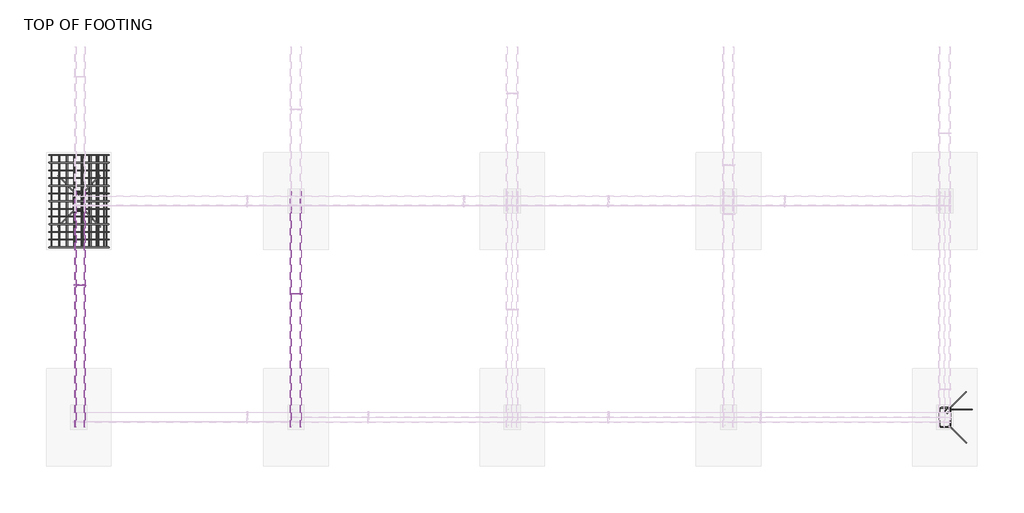
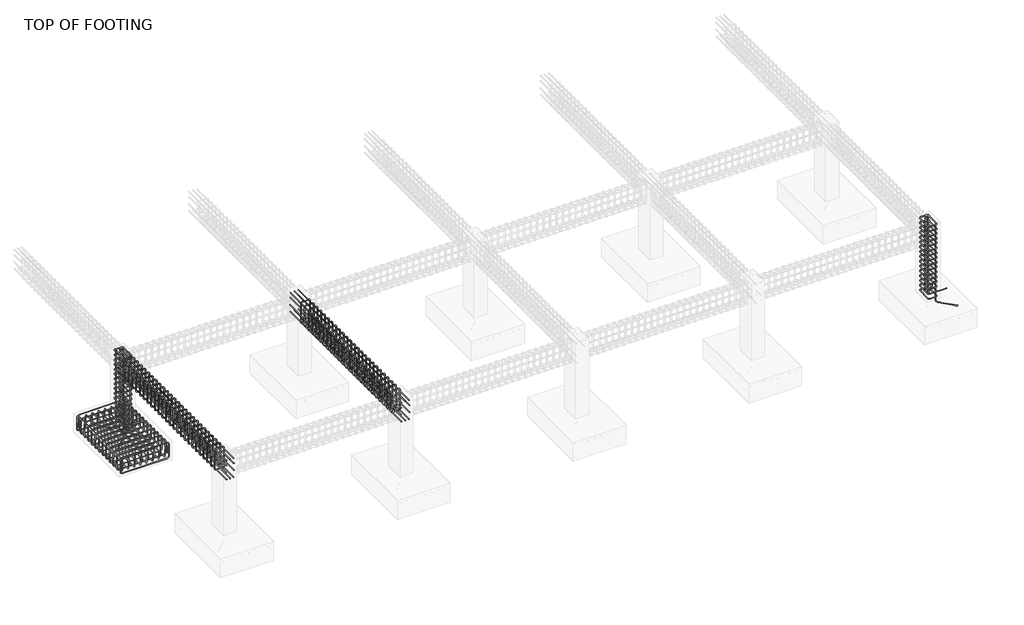
# One storey, part 5 of 21: 28 reinforcing bars.
"""IFC4 building model written with IfcOpenShell, lengths in millimetres."""

from ifc_helpers import new_model, si_unit, point, frame, origin, place, context, project, spatial, polyline, circle_curve, trimmed, segment, composite_curve, source, transform, mapped, element, save
from ifc_brep_helpers import swept_disk

model = new_model("IFC4")

# Units and contexts
model_context = context("Model", 3, world=origin())
ifc_project = project(units=[si_unit("LENGTHUNIT", "METRE", prefix="MILLI")], contexts=[model_context])

# Site, building, storey
site = spatial("IfcSite", under=ifc_project)
building = spatial("IfcBuilding", under=site)
storey = spatial("IfcBuildingStorey", under=building, Name="TOP OF FOOTING", Elevation=-1828.8)

# Reinforcing bars
placement = place(None, origin())
reinforcing_bar_shape = source(origin(), model_context, "Body", "SolidModel", [
    swept_disk(composite_curve([segment(polyline([(-13268.2584825, 4443.1886958, -2045.4168622), (-13268.2584825, 4443.1886958, -2192.7168622)]), True, "CONTINUOUS"), segment(trimmed(circle_curve(frame((-13314.6084825, 4443.1886958, -2192.7168622), z_axis=(0.0, 1.0, 0.0), x_axis=(46.350000000000364, 0.0, 0.0)), 46.35), [point((-13268.2584825, 4443.1886958, -2192.7168622))], [point((-13314.6084825, 4443.1886958, -2239.0668622))], True, "CARTESIAN"), True, "CONTINUOUS"), segment(polyline([(-13314.6084825, 4443.1886958, -2239.0668622), (-14329.2084825, 4443.1886958, -2239.0668622)]), True, "CONTINUOUS"), segment(trimmed(circle_curve(frame((-14329.2084825, 4443.1886958, -2192.7168622), z_axis=(0.0, 1.0, 0.0), x_axis=(0.0, 0.0, -46.34999999999991)), 46.35), [point((-14329.2084825, 4443.1886958, -2239.0668622))], [point((-14375.5584825, 4443.1886958, -2192.7168622))], True, "CARTESIAN"), True, "CONTINUOUS"), segment(polyline([(-14375.5584825, 4443.1886958, -2192.7168622), (-14375.5584825, 4443.1886958, -2045.4168622)]), True, "CONTINUOUS")], self_intersect=False), 6.35),
])
element("IfcReinforcingBar", 1, at=placement, inside=storey, context=model_context, shape_type="MappedRepresentation", body=[
    mapped(reinforcing_bar_shape, transform((0.0, 0.0, 0.0), x_axis=(1.0, 0.0, 0.0), y_axis=(0.0, 1.0, 0.0), z_axis=(0.0, 0.0, 1.0))),
    mapped(reinforcing_bar_shape, transform((0.0, -142.275, 0.0), x_axis=(1.0, 0.0, 0.0), y_axis=(0.0, 1.0, 0.0), z_axis=(0.0, 0.0, 1.0))),
    mapped(reinforcing_bar_shape, transform((0.0, -284.55, 0.0), x_axis=(1.0, 0.0, 0.0), y_axis=(0.0, 1.0, 0.0), z_axis=(0.0, 0.0, 1.0))),
    mapped(reinforcing_bar_shape, transform((0.0, -426.825, 0.0), x_axis=(1.0, 0.0, 0.0), y_axis=(0.0, 1.0, 0.0), z_axis=(0.0, 0.0, 1.0))),
    mapped(reinforcing_bar_shape, transform((0.0, -569.1, 0.0), x_axis=(1.0, 0.0, 0.0), y_axis=(0.0, 1.0, 0.0), z_axis=(0.0, 0.0, 1.0))),
    mapped(reinforcing_bar_shape, transform((0.0, -711.375, 0.0), x_axis=(1.0, 0.0, 0.0), y_axis=(0.0, 1.0, 0.0), z_axis=(0.0, 0.0, 1.0))),
    mapped(reinforcing_bar_shape, transform((0.0, -853.65, 0.0), x_axis=(1.0, 0.0, 0.0), y_axis=(0.0, 1.0, 0.0), z_axis=(0.0, 0.0, 1.0))),
    mapped(reinforcing_bar_shape, transform((0.0, -995.925, 0.0), x_axis=(1.0, 0.0, 0.0), y_axis=(0.0, 1.0, 0.0), z_axis=(0.0, 0.0, 1.0))),
    mapped(reinforcing_bar_shape, transform((0.0, -1138.2, 0.0), x_axis=(1.0, 0.0, 0.0), y_axis=(0.0, 1.0, 0.0), z_axis=(0.0, 0.0, 1.0))),
    mapped(reinforcing_bar_shape, transform((0.0, -1280.475, 0.0), x_axis=(1.0, 0.0, 0.0), y_axis=(0.0, 1.0, 0.0), z_axis=(0.0, 0.0, 1.0))),
    mapped(reinforcing_bar_shape, transform((0.0, -1422.75, 0.0), x_axis=(1.0, 0.0, 0.0), y_axis=(0.0, 1.0, 0.0), z_axis=(0.0, 0.0, 1.0))),
    mapped(reinforcing_bar_shape, transform((0.0, -1565.025, 0.0), x_axis=(1.0, 0.0, 0.0), y_axis=(0.0, 1.0, 0.0), z_axis=(0.0, 0.0, 1.0))),
    mapped(reinforcing_bar_shape, transform((0.0, -1707.3, 0.0), x_axis=(1.0, 0.0, 0.0), y_axis=(0.0, 1.0, 0.0), z_axis=(0.0, 0.0, 1.0))),
])
reinforcing_bar_2_shape = source(origin(), model_context, "Body", "SolidModel", [
    swept_disk(composite_curve([segment(polyline([(-14372.2274202, 4443.1886958, -2057.1074344), (-14372.2274202, 4443.1886958, -1909.8074344)]), True, "CONTINUOUS"), segment(trimmed(circle_curve(frame((-14325.8774202, 4443.1886958, -1909.8074344), z_axis=(0.0, 1.0, 0.0), x_axis=(-46.350000000000364, 0.0, 0.0)), 46.35), [point((-14372.2274202, 4443.1886958, -1909.8074344))], [point((-14325.8774202, 4443.1886958, -1863.4574344))], True, "CARTESIAN"), True, "CONTINUOUS"), segment(polyline([(-14325.8774202, 4443.1886958, -1863.4574344), (-13316.98705, 4443.1886958, -1863.4574344)]), True, "CONTINUOUS"), segment(trimmed(circle_curve(frame((-13316.98705, 4443.1886958, -1909.8074344), z_axis=(0.0, 1.0, 0.0), x_axis=(0.0, 0.0, 46.34999999999991)), 46.35), [point((-13316.98705, 4443.1886958, -1863.4574344))], [point((-13270.63705, 4443.1886958, -1909.8074344))], True, "CARTESIAN"), True, "CONTINUOUS"), segment(polyline([(-13270.63705, 4443.1886958, -1909.8074344), (-13270.63705, 4443.1886958, -2057.1074344)]), True, "CONTINUOUS")], self_intersect=False), 6.35),
])
element("IfcReinforcingBar", 2, at=placement, inside=storey, context=model_context, shape_type="MappedRepresentation", body=[
    mapped(reinforcing_bar_2_shape, transform((0.0, 0.0, 0.0), x_axis=(1.0, 0.0, 0.0), y_axis=(0.0, 1.0, 0.0), z_axis=(0.0, 0.0, 1.0))),
    mapped(reinforcing_bar_2_shape, transform((0.0, -142.275, 0.0), x_axis=(1.0, 0.0, 0.0), y_axis=(0.0, 1.0, 0.0), z_axis=(0.0, 0.0, 1.0))),
    mapped(reinforcing_bar_2_shape, transform((0.0, -284.55, 0.0), x_axis=(1.0, 0.0, 0.0), y_axis=(0.0, 1.0, 0.0), z_axis=(0.0, 0.0, 1.0))),
    mapped(reinforcing_bar_2_shape, transform((0.0, -426.825, 0.0), x_axis=(1.0, 0.0, 0.0), y_axis=(0.0, 1.0, 0.0), z_axis=(0.0, 0.0, 1.0))),
    mapped(reinforcing_bar_2_shape, transform((0.0, -569.1, 0.0), x_axis=(1.0, 0.0, 0.0), y_axis=(0.0, 1.0, 0.0), z_axis=(0.0, 0.0, 1.0))),
    mapped(reinforcing_bar_2_shape, transform((0.0, -711.375, 0.0), x_axis=(1.0, 0.0, 0.0), y_axis=(0.0, 1.0, 0.0), z_axis=(0.0, 0.0, 1.0))),
    mapped(reinforcing_bar_2_shape, transform((0.0, -853.65, 0.0), x_axis=(1.0, 0.0, 0.0), y_axis=(0.0, 1.0, 0.0), z_axis=(0.0, 0.0, 1.0))),
    mapped(reinforcing_bar_2_shape, transform((0.0, -995.925, 0.0), x_axis=(1.0, 0.0, 0.0), y_axis=(0.0, 1.0, 0.0), z_axis=(0.0, 0.0, 1.0))),
    mapped(reinforcing_bar_2_shape, transform((0.0, -1138.2, 0.0), x_axis=(1.0, 0.0, 0.0), y_axis=(0.0, 1.0, 0.0), z_axis=(0.0, 0.0, 1.0))),
    mapped(reinforcing_bar_2_shape, transform((0.0, -1280.475, 0.0), x_axis=(1.0, 0.0, 0.0), y_axis=(0.0, 1.0, 0.0), z_axis=(0.0, 0.0, 1.0))),
    mapped(reinforcing_bar_2_shape, transform((0.0, -1422.75, 0.0), x_axis=(1.0, 0.0, 0.0), y_axis=(0.0, 1.0, 0.0), z_axis=(0.0, 0.0, 1.0))),
    mapped(reinforcing_bar_2_shape, transform((0.0, -1565.025, 0.0), x_axis=(1.0, 0.0, 0.0), y_axis=(0.0, 1.0, 0.0), z_axis=(0.0, 0.0, 1.0))),
    mapped(reinforcing_bar_2_shape, transform((0.0, -1707.3, 0.0), x_axis=(1.0, 0.0, 0.0), y_axis=(0.0, 1.0, 0.0), z_axis=(0.0, 0.0, 1.0))),
])
reinforcing_bar_3_shape = source(origin(), model_context, "Body", "SolidModel", [
    swept_disk(composite_curve([segment(polyline([(-13314.2120502, 4443.1886958, -2099.3509187), (-13314.2120502, 4443.1886958, -1952.0509187)]), True, "CONTINUOUS"), segment(trimmed(circle_curve(frame((-13314.2120502, 4396.8386958, -1952.0509187), z_axis=(1.0, 0.0, 0.0), x_axis=(0.0, 46.349999999999454, 0.0)), 46.35), [point((-13314.2120502, 4443.1886958, -1952.0509187))], [point((-13314.2120502, 4396.8386958, -1905.7009187))], True, "CARTESIAN"), True, "CONTINUOUS"), segment(polyline([(-13314.2120502, 4396.8386958, -1905.7009187), (-13314.2120502, 2782.2386958, -1905.7009187)]), True, "CONTINUOUS"), segment(trimmed(circle_curve(frame((-13314.2120502, 2782.2386958, -1952.0509187), z_axis=(1.0, 0.0, 0.0), x_axis=(0.0, 0.0, 46.34999999999991)), 46.35), [point((-13314.2120502, 2782.2386958, -1905.7009187))], [point((-13314.2120502, 2735.8886958, -1952.0509187))], True, "CARTESIAN"), True, "CONTINUOUS"), segment(polyline([(-13314.2120502, 2735.8886958, -1952.0509187), (-13314.2120502, 2735.8886958, -2099.3509187)]), True, "CONTINUOUS")], self_intersect=False), 6.35),
])
element("IfcReinforcingBar", 3, at=placement, inside=storey, context=model_context, shape_type="MappedRepresentation", body=[
    mapped(reinforcing_bar_3_shape, transform((0.0, 0.0, 0.0), x_axis=(1.0, 0.0, 0.0), y_axis=(0.0, 1.0, 0.0), z_axis=(0.0, 0.0, 1.0))),
    mapped(reinforcing_bar_3_shape, transform((-145.0295561, 0.0, 0.0), x_axis=(1.0, 0.0, 0.0), y_axis=(0.0, 1.0, 0.0), z_axis=(0.0, 0.0, 1.0))),
    mapped(reinforcing_bar_3_shape, transform((-290.0591123, 0.0, 0.0), x_axis=(1.0, 0.0, 0.0), y_axis=(0.0, 1.0, 0.0), z_axis=(0.0, 0.0, 1.0))),
    mapped(reinforcing_bar_3_shape, transform((-435.0886684, 0.0, 0.0), x_axis=(1.0, 0.0, 0.0), y_axis=(0.0, 1.0, 0.0), z_axis=(0.0, 0.0, 1.0))),
    mapped(reinforcing_bar_3_shape, transform((-580.1182245, 0.0, 0.0), x_axis=(1.0, 0.0, 0.0), y_axis=(0.0, 1.0, 0.0), z_axis=(0.0, 0.0, 1.0))),
    mapped(reinforcing_bar_3_shape, transform((-725.1477807, 0.0, 0.0), x_axis=(1.0, 0.0, 0.0), y_axis=(0.0, 1.0, 0.0), z_axis=(0.0, 0.0, 1.0))),
    mapped(reinforcing_bar_3_shape, transform((-870.1773368, 0.0, 0.0), x_axis=(1.0, 0.0, 0.0), y_axis=(0.0, 1.0, 0.0), z_axis=(0.0, 0.0, 1.0))),
    mapped(reinforcing_bar_3_shape, transform((-1015.206893, 0.0, 0.0), x_axis=(1.0, 0.0, 0.0), y_axis=(0.0, 1.0, 0.0), z_axis=(0.0, 0.0, 1.0))),
])
reinforcing_bar_4_shape = source(origin(), model_context, "Body", "SolidModel", [
    swept_disk(composite_curve([segment(polyline([(-14329.4189432, 4443.1886958, -2006.0306816), (-14329.4189432, 4443.1886958, -2153.3306816)]), True, "CONTINUOUS"), segment(trimmed(circle_curve(frame((-14329.4189432, 4396.8386958, -2153.3306816), z_axis=(-1.0, 0.0, 0.0), x_axis=(0.0, 46.349999999999454, 0.0)), 46.35), [point((-14329.4189432, 4443.1886958, -2153.3306816))], [point((-14329.4189432, 4396.8386958, -2199.6806816))], True, "CARTESIAN"), True, "CONTINUOUS"), segment(polyline([(-14329.4189432, 4396.8386958, -2199.6806816), (-14329.4189432, 2782.2386958, -2199.6806816)]), True, "CONTINUOUS"), segment(trimmed(circle_curve(frame((-14329.4189432, 2782.2386958, -2153.3306816), z_axis=(-1.0, 0.0, 0.0), x_axis=(0.0, 0.0, -46.34999999999991)), 46.35), [point((-14329.4189432, 2782.2386958, -2199.6806816))], [point((-14329.4189432, 2735.8886958, -2153.3306816))], True, "CARTESIAN"), True, "CONTINUOUS"), segment(polyline([(-14329.4189432, 2735.8886958, -2153.3306816), (-14329.4189432, 2735.8886958, -2006.0306816)]), True, "CONTINUOUS")], self_intersect=False), 6.35),
])
element("IfcReinforcingBar", 4, at=placement, inside=storey, context=model_context, shape_type="MappedRepresentation", body=[
    mapped(reinforcing_bar_4_shape, transform((0.0, 0.0, 0.0), x_axis=(1.0, 0.0, 0.0), y_axis=(0.0, 1.0, 0.0), z_axis=(0.0, 0.0, 1.0))),
    mapped(reinforcing_bar_4_shape, transform((138.8823255, 0.0, 0.0), x_axis=(1.0, 0.0, 0.0), y_axis=(0.0, 1.0, 0.0), z_axis=(0.0, 0.0, 1.0))),
    mapped(reinforcing_bar_4_shape, transform((277.7646509, 0.0, 0.0), x_axis=(1.0, 0.0, 0.0), y_axis=(0.0, 1.0, 0.0), z_axis=(0.0, 0.0, 1.0))),
    mapped(reinforcing_bar_4_shape, transform((416.6469764, 0.0, 0.0), x_axis=(1.0, 0.0, 0.0), y_axis=(0.0, 1.0, 0.0), z_axis=(0.0, 0.0, 1.0))),
    mapped(reinforcing_bar_4_shape, transform((555.5293018, 0.0, 0.0), x_axis=(1.0, 0.0, 0.0), y_axis=(0.0, 1.0, 0.0), z_axis=(0.0, 0.0, 1.0))),
    mapped(reinforcing_bar_4_shape, transform((694.4116273, 0.0, 0.0), x_axis=(1.0, 0.0, 0.0), y_axis=(0.0, 1.0, 0.0), z_axis=(0.0, 0.0, 1.0))),
    mapped(reinforcing_bar_4_shape, transform((833.2939527, 0.0, 0.0), x_axis=(1.0, 0.0, 0.0), y_axis=(0.0, 1.0, 0.0), z_axis=(0.0, 0.0, 1.0))),
    mapped(reinforcing_bar_4_shape, transform((972.1762782, 0.0, 0.0), x_axis=(1.0, 0.0, 0.0), y_axis=(0.0, 1.0, 0.0), z_axis=(0.0, 0.0, 1.0))),
])
reinforcing_bar_5_shape = source(origin(), model_context, "Body", "SolidModel", [
    swept_disk(composite_curve([segment(polyline([(-13827.5198431, 3703.2629305, -46.35), (-13771.7762801, 3759.0064934, -46.35)]), True, "CONTINUOUS"), segment(trimmed(circle_curve(frame((-13749.6084825, 3736.8386958, -46.35), z_axis=(0.0, 0.0, -1.0), x_axis=(-22.167797600000995, 22.167797600000085, 0.0)), 31.35), [point((-13771.7762801, 3759.0064934, -46.35))], [point((-13718.2584825, 3736.8386958, -46.35))], True, "CARTESIAN"), True, "CONTINUOUS"), segment(polyline([(-13718.2584825, 3736.8386958, -46.35), (-13718.2584825, 3442.2386958, -46.35)]), True, "CONTINUOUS"), segment(trimmed(circle_curve(frame((-13749.6084825, 3442.2386958, -46.35), z_axis=(0.0, 0.0, -1.0), x_axis=(31.350000000000364, 0.0, 0.0)), 31.35), [point((-13718.2584825, 3442.2386958, -46.35))], [point((-13749.6084825, 3410.8886958, -46.35))], True, "CARTESIAN"), True, "CONTINUOUS"), segment(polyline([(-13749.6084825, 3410.8886958, -46.35), (-13894.2084825, 3410.8886958, -46.35)]), True, "CONTINUOUS"), segment(trimmed(circle_curve(frame((-13894.2084825, 3442.2189107, -45.2363875), z_axis=(0.0, 0.035521928334481916, -0.9993688971583016), x_axis=(0.0, -31.3302149000001, -1.1136125000000021)), 31.35), [point((-13894.2084825, 3410.8886958, -46.35))], [point((-13925.5584825, 3442.2189107, -45.2363875))], True, "CARTESIAN"), True, "CONTINUOUS"), segment(polyline([(-13925.5584825, 3442.2189107, -45.2363875), (-13925.5584825, 3736.8584809, -34.7636125)]), True, "CONTINUOUS"), segment(trimmed(circle_curve(frame((-13894.2084825, 3736.8584809, -34.7636125), z_axis=(0.0, 0.035521928334481916, -0.9993688971583016), x_axis=(-31.350000000000364, 0.0, 0.0)), 31.35), [point((-13925.5584825, 3736.8584809, -34.7636125))], [point((-13894.2084825, 3768.1886958, -33.65))], True, "CARTESIAN"), True, "CONTINUOUS"), segment(polyline([(-13894.2084825, 3768.1886958, -33.65), (-13749.6084825, 3768.1886958, -33.65)]), True, "CONTINUOUS"), segment(trimmed(circle_curve(frame((-13749.6084825, 3736.8386958, -33.65), z_axis=(0.0, 0.0, -1.0), x_axis=(0.0, 31.34999999999991, 0.0)), 31.35), [point((-13749.6084825, 3768.1886958, -33.65))], [point((-13727.4406849, 3714.6708982, -33.65))], True, "CARTESIAN"), True, "CONTINUOUS"), segment(polyline([(-13727.4406849, 3714.6708982, -33.65), (-13783.1842479, 3658.9273353, -33.65)]), True, "CONTINUOUS")], self_intersect=False), 6.35),
])
element("IfcReinforcingBar", 5, at=placement, inside=storey, context=model_context, shape_type="MappedRepresentation", body=[
    mapped(reinforcing_bar_5_shape, transform((0.0, 0.0, 0.0), x_axis=(1.0, 0.0, 0.0), y_axis=(0.0, 1.0, 0.0), z_axis=(0.0, 0.0, 1.0))),
    mapped(reinforcing_bar_5_shape, transform((0.0, 0.0, -115.74), x_axis=(1.0, 0.0, 0.0), y_axis=(0.0, 1.0, 0.0), z_axis=(0.0, 0.0, 1.0))),
    mapped(reinforcing_bar_5_shape, transform((0.0, 0.0, -231.48), x_axis=(1.0, 0.0, 0.0), y_axis=(0.0, 1.0, 0.0), z_axis=(0.0, 0.0, 1.0))),
    mapped(reinforcing_bar_5_shape, transform((0.0, 0.0, -347.22), x_axis=(1.0, 0.0, 0.0), y_axis=(0.0, 1.0, 0.0), z_axis=(0.0, 0.0, 1.0))),
    mapped(reinforcing_bar_5_shape, transform((0.0, 0.0, -462.96), x_axis=(1.0, 0.0, 0.0), y_axis=(0.0, 1.0, 0.0), z_axis=(0.0, 0.0, 1.0))),
    mapped(reinforcing_bar_5_shape, transform((0.0, 0.0, -578.7), x_axis=(1.0, 0.0, 0.0), y_axis=(0.0, 1.0, 0.0), z_axis=(0.0, 0.0, 1.0))),
    mapped(reinforcing_bar_5_shape, transform((0.0, 0.0, -694.44), x_axis=(1.0, 0.0, 0.0), y_axis=(0.0, 1.0, 0.0), z_axis=(0.0, 0.0, 1.0))),
    mapped(reinforcing_bar_5_shape, transform((0.0, 0.0, -810.18), x_axis=(1.0, 0.0, 0.0), y_axis=(0.0, 1.0, 0.0), z_axis=(0.0, 0.0, 1.0))),
    mapped(reinforcing_bar_5_shape, transform((0.0, 0.0, -925.92), x_axis=(1.0, 0.0, 0.0), y_axis=(0.0, 1.0, 0.0), z_axis=(0.0, 0.0, 1.0))),
    mapped(reinforcing_bar_5_shape, transform((0.0, 0.0, -1041.66), x_axis=(1.0, 0.0, 0.0), y_axis=(0.0, 1.0, 0.0), z_axis=(0.0, 0.0, 1.0))),
    mapped(reinforcing_bar_5_shape, transform((0.0, 0.0, -1157.4), x_axis=(1.0, 0.0, 0.0), y_axis=(0.0, 1.0, 0.0), z_axis=(0.0, 0.0, 1.0))),
    mapped(reinforcing_bar_5_shape, transform((0.0, 0.0, -1273.14), x_axis=(1.0, 0.0, 0.0), y_axis=(0.0, 1.0, 0.0), z_axis=(0.0, 0.0, 1.0))),
    mapped(reinforcing_bar_5_shape, transform((0.0, 0.0, -1388.88), x_axis=(1.0, 0.0, 0.0), y_axis=(0.0, 1.0, 0.0), z_axis=(0.0, 0.0, 1.0))),
    mapped(reinforcing_bar_5_shape, transform((0.0, 0.0, -1504.62), x_axis=(1.0, 0.0, 0.0), y_axis=(0.0, 1.0, 0.0), z_axis=(0.0, 0.0, 1.0))),
    mapped(reinforcing_bar_5_shape, transform((0.0, 0.0, -1620.36), x_axis=(1.0, 0.0, 0.0), y_axis=(0.0, 1.0, 0.0), z_axis=(0.0, 0.0, 1.0))),
    mapped(reinforcing_bar_5_shape, transform((0.0, 0.0, -1736.1), x_axis=(1.0, 0.0, 0.0), y_axis=(0.0, 1.0, 0.0), z_axis=(0.0, 0.0, 1.0))),
])
element("IfcReinforcingBar", 6, at=placement, inside=storey, context=model_context, shape_type="SolidModel", body=[
    swept_disk(composite_curve([segment(polyline([(-13750.0878823, 3737.940488, -40.0), (-13750.0878823, 3737.940488, -1882.5259187)]), True, "CONTINUOUS"), segment(trimmed(circle_curve(frame((-13703.7378823, 3737.940488, -1882.5259187), z_axis=(0.0, -1.0, 0.0), x_axis=(-46.350000000000364, 0.0, 0.0)), 46.35), [point((-13750.0878823, 3737.940488, -1882.5259187))], [point((-13703.7378823, 3737.940488, -1928.8759187))], True, "CARTESIAN"), True, "CONTINUOUS"), segment(polyline([(-13703.7378823, 3737.940488, -1928.8759187), (-13314.2120502, 3737.940488, -1928.8759187)]), True, "CONTINUOUS")], self_intersect=False), 6.35),
])
element("IfcReinforcingBar", 7, at=placement, inside=storey, context=model_context, shape_type="SolidModel", body=[
    swept_disk(composite_curve([segment(polyline([(-13750.0878823, 3737.940488, -40.0), (-13750.0878823, 3737.940488, -1882.5259187)]), True, "CONTINUOUS"), segment(trimmed(circle_curve(frame((-13717.6297647, 3771.0281458, -1882.5259187), z_axis=(0.7138653253877265, -0.7002830122236834, 0.0), x_axis=(-32.45811760000106, -33.08765779999976, 0.0)), 46.35), [point((-13750.0878823, 3737.940488, -1882.5259187))], [point((-13717.6297647, 3771.0281458, -1928.8759187))], True, "CARTESIAN"), True, "CONTINUOUS"), segment(polyline([(-13717.6297647, 3771.0281458, -1928.8759187), (-13432.8602442, 4061.320903, -1928.8759187)]), True, "CONTINUOUS")], self_intersect=False), 6.35),
])
element("IfcReinforcingBar", 8, at=placement, inside=storey, context=model_context, shape_type="SolidModel", body=[
    swept_disk(composite_curve([segment(polyline([(-13893.7290828, 3737.940488, -40.0), (-13893.7290828, 3737.940488, -1882.5259187)]), True, "CONTINUOUS"), segment(trimmed(circle_curve(frame((-13926.1872004, 3771.0281458, -1882.5259187), z_axis=(0.7138653253877091, 0.700283012223701, 0.0), x_axis=(32.45811759999924, -33.08765779999976, 0.0)), 46.35), [point((-13893.7290828, 3737.940488, -1882.5259187))], [point((-13926.1872004, 3771.0281458, -1928.8759187))], True, "CARTESIAN"), True, "CONTINUOUS"), segment(polyline([(-13926.1872004, 3771.0281458, -1928.8759187), (-14210.9567208, 4061.320903, -1928.8759187)]), True, "CONTINUOUS")], self_intersect=False), 6.35),
])
element("IfcReinforcingBar", 9, at=placement, inside=storey, context=model_context, shape_type="SolidModel", body=[
    swept_disk(composite_curve([segment(polyline([(-13745.0878823, 3438.6369036, -40.0), (-13745.0878823, 3438.6369036, -1882.5259187)]), True, "CONTINUOUS"), segment(trimmed(circle_curve(frame((-13712.6297647, 3405.5492458, -1882.5259187), z_axis=(-0.7138653253877265, -0.7002830122236834, 0.0), x_axis=(-32.45811760000106, 33.087657800000216, 0.0)), 46.35), [point((-13745.0878823, 3438.6369036, -1882.5259187))], [point((-13712.6297647, 3405.5492458, -1928.8759187))], True, "CARTESIAN"), True, "CONTINUOUS"), segment(polyline([(-13712.6297647, 3405.5492458, -1928.8759187), (-13427.8602442, 3115.2564887, -1928.8759187)]), True, "CONTINUOUS")], self_intersect=False), 6.35),
])
element("IfcReinforcingBar", 10, at=placement, inside=storey, context=model_context, shape_type="SolidModel", body=[
    swept_disk(composite_curve([segment(polyline([(-13893.7290828, 3441.1369036, -40.0), (-13893.7290828, 3441.1369036, -1882.5259187)]), True, "CONTINUOUS"), segment(trimmed(circle_curve(frame((-13926.1872004, 3408.0492458, -1882.5259187), z_axis=(-0.7138653253877092, 0.7002830122237009, 0.0), x_axis=(32.45811759999924, 33.087657800000216, 0.0)), 46.35), [point((-13893.7290828, 3441.1369036, -1882.5259187))], [point((-13926.1872004, 3408.0492458, -1928.8759187))], True, "CARTESIAN"), True, "CONTINUOUS"), segment(polyline([(-13926.1872004, 3408.0492458, -1928.8759187), (-14210.9567208, 3117.7564887, -1928.8759187)]), True, "CONTINUOUS")], self_intersect=False), 6.35),
])
reinforcing_bar_6_shape = source(origin(), model_context, "Body", "SolidModel", [
    swept_disk(composite_curve([segment(polyline([(2192.2072855, -296.7370695, -46.35), (2247.9508485, -240.9935066, -46.35)]), True, "CONTINUOUS"), segment(trimmed(circle_curve(frame((2270.1186461, -263.1613042, -46.35), z_axis=(0.0, 0.0, -1.0), x_axis=(-22.167797600000085, 22.16779760000003, 0.0)), 31.35), [point((2247.9508485, -240.9935066, -46.35))], [point((2301.4686461, -263.1613042, -46.35))], True, "CARTESIAN"), True, "CONTINUOUS"), segment(polyline([(2301.4686461, -263.1613042, -46.35), (2301.4686461, -557.7613042, -46.35)]), True, "CONTINUOUS"), segment(trimmed(circle_curve(frame((2270.1186461, -557.7613042, -46.35), z_axis=(0.0, 0.0, -1.0), x_axis=(31.34999999999991, 0.0, 0.0)), 31.35), [point((2301.4686461, -557.7613042, -46.35))], [point((2270.1186461, -589.1113042, -46.35))], True, "CARTESIAN"), True, "CONTINUOUS"), segment(polyline([(2270.1186461, -589.1113042, -46.35), (2125.5186461, -589.1113042, -46.35)]), True, "CONTINUOUS"), segment(trimmed(circle_curve(frame((2125.5186461, -557.7810893, -45.2363875), z_axis=(0.0, 0.035521928334481916, -0.9993688971583016), x_axis=(0.0, -31.330214899999987, -1.1136125000000021)), 31.35), [point((2125.5186461, -589.1113042, -46.35))], [point((2094.1686461, -557.7810893, -45.2363875))], True, "CARTESIAN"), True, "CONTINUOUS"), segment(polyline([(2094.1686461, -557.7810893, -45.2363875), (2094.1686461, -263.1415191, -34.7636125)]), True, "CONTINUOUS"), segment(trimmed(circle_curve(frame((2125.5186461, -263.1415191, -34.7636125), z_axis=(0.0, 0.035521928334481916, -0.9993688971583016), x_axis=(-31.34999999999991, 0.0, 0.0)), 31.35), [point((2094.1686461, -263.1415191, -34.7636125))], [point((2125.5186461, -231.8113042, -33.65))], True, "CARTESIAN"), True, "CONTINUOUS"), segment(polyline([(2125.5186461, -231.8113042, -33.65), (2270.1186461, -231.8113042, -33.65)]), True, "CONTINUOUS"), segment(trimmed(circle_curve(frame((2270.1186461, -263.1613042, -33.65), z_axis=(0.0, 0.0, -1.0), x_axis=(0.0, 31.350000000000023, 0.0)), 31.35), [point((2270.1186461, -231.8113042, -33.65))], [point((2292.2864437, -285.3291018, -33.65))], True, "CARTESIAN"), True, "CONTINUOUS"), segment(polyline([(2292.2864437, -285.3291018, -33.65), (2236.5428807, -341.0726647, -33.65)]), True, "CONTINUOUS")], self_intersect=False), 6.35),
])
element("IfcReinforcingBar", 11, at=placement, inside=storey, context=model_context, shape_type="MappedRepresentation", body=[
    mapped(reinforcing_bar_6_shape, transform((0.0, 0.0, 0.0), x_axis=(1.0, 0.0, 0.0), y_axis=(0.0, 1.0, 0.0), z_axis=(0.0, 0.0, 1.0))),
    mapped(reinforcing_bar_6_shape, transform((0.0, 0.0, -115.74), x_axis=(1.0, 0.0, 0.0), y_axis=(0.0, 1.0, 0.0), z_axis=(0.0, 0.0, 1.0))),
    mapped(reinforcing_bar_6_shape, transform((0.0, 0.0, -231.48), x_axis=(1.0, 0.0, 0.0), y_axis=(0.0, 1.0, 0.0), z_axis=(0.0, 0.0, 1.0))),
    mapped(reinforcing_bar_6_shape, transform((0.0, 0.0, -347.22), x_axis=(1.0, 0.0, 0.0), y_axis=(0.0, 1.0, 0.0), z_axis=(0.0, 0.0, 1.0))),
    mapped(reinforcing_bar_6_shape, transform((0.0, 0.0, -462.96), x_axis=(1.0, 0.0, 0.0), y_axis=(0.0, 1.0, 0.0), z_axis=(0.0, 0.0, 1.0))),
    mapped(reinforcing_bar_6_shape, transform((0.0, 0.0, -578.7), x_axis=(1.0, 0.0, 0.0), y_axis=(0.0, 1.0, 0.0), z_axis=(0.0, 0.0, 1.0))),
    mapped(reinforcing_bar_6_shape, transform((0.0, 0.0, -694.44), x_axis=(1.0, 0.0, 0.0), y_axis=(0.0, 1.0, 0.0), z_axis=(0.0, 0.0, 1.0))),
    mapped(reinforcing_bar_6_shape, transform((0.0, 0.0, -810.18), x_axis=(1.0, 0.0, 0.0), y_axis=(0.0, 1.0, 0.0), z_axis=(0.0, 0.0, 1.0))),
    mapped(reinforcing_bar_6_shape, transform((0.0, 0.0, -925.92), x_axis=(1.0, 0.0, 0.0), y_axis=(0.0, 1.0, 0.0), z_axis=(0.0, 0.0, 1.0))),
    mapped(reinforcing_bar_6_shape, transform((0.0, 0.0, -1041.66), x_axis=(1.0, 0.0, 0.0), y_axis=(0.0, 1.0, 0.0), z_axis=(0.0, 0.0, 1.0))),
    mapped(reinforcing_bar_6_shape, transform((0.0, 0.0, -1157.4), x_axis=(1.0, 0.0, 0.0), y_axis=(0.0, 1.0, 0.0), z_axis=(0.0, 0.0, 1.0))),
    mapped(reinforcing_bar_6_shape, transform((0.0, 0.0, -1273.14), x_axis=(1.0, 0.0, 0.0), y_axis=(0.0, 1.0, 0.0), z_axis=(0.0, 0.0, 1.0))),
    mapped(reinforcing_bar_6_shape, transform((0.0, 0.0, -1388.88), x_axis=(1.0, 0.0, 0.0), y_axis=(0.0, 1.0, 0.0), z_axis=(0.0, 0.0, 1.0))),
    mapped(reinforcing_bar_6_shape, transform((0.0, 0.0, -1504.62), x_axis=(1.0, 0.0, 0.0), y_axis=(0.0, 1.0, 0.0), z_axis=(0.0, 0.0, 1.0))),
    mapped(reinforcing_bar_6_shape, transform((0.0, 0.0, -1620.36), x_axis=(1.0, 0.0, 0.0), y_axis=(0.0, 1.0, 0.0), z_axis=(0.0, 0.0, 1.0))),
    mapped(reinforcing_bar_6_shape, transform((0.0, 0.0, -1736.1), x_axis=(1.0, 0.0, 0.0), y_axis=(0.0, 1.0, 0.0), z_axis=(0.0, 0.0, 1.0))),
])
element("IfcReinforcingBar", 12, at=placement, inside=storey, context=model_context, shape_type="SolidModel", body=[
    swept_disk(composite_curve([segment(polyline([(2269.6392463, -262.059512, -40.0), (2269.6392463, -262.059512, -1882.5259187)]), True, "CONTINUOUS"), segment(trimmed(circle_curve(frame((2315.9892463, -262.059512, -1882.5259187), z_axis=(0.0, -1.0, 0.0), x_axis=(-46.34999999999991, 0.0, 0.0)), 46.35), [point((2269.6392463, -262.059512, -1882.5259187))], [point((2315.9892463, -262.059512, -1928.8759187))], True, "CARTESIAN"), True, "CONTINUOUS"), segment(polyline([(2315.9892463, -262.059512, -1928.8759187), (2705.5150784, -262.059512, -1928.8759187)]), True, "CONTINUOUS")], self_intersect=False), 6.35),
])
element("IfcReinforcingBar", 13, at=placement, inside=storey, context=model_context, shape_type="SolidModel", body=[
    swept_disk(composite_curve([segment(polyline([(2269.6392463, -262.059512, -40.0), (2269.6392463, -262.059512, -1882.5259187)]), True, "CONTINUOUS"), segment(trimmed(circle_curve(frame((2302.0973639, -228.9718542, -1882.5259187), z_axis=(0.7138653253877265, -0.7002830122236834, 0.0), x_axis=(-32.458117599999696, -33.08765779999999, 0.0)), 46.35), [point((2269.6392463, -262.059512, -1882.5259187))], [point((2302.0973639, -228.9718542, -1928.8759187))], True, "CARTESIAN"), True, "CONTINUOUS"), segment(polyline([(2302.0973639, -228.9718542, -1928.8759187), (2586.8668844, 61.320903, -1928.8759187)]), True, "CONTINUOUS")], self_intersect=False), 6.35),
])
element("IfcReinforcingBar", 14, at=placement, inside=storey, context=model_context, shape_type="SolidModel", body=[
    swept_disk(composite_curve([segment(polyline([(2274.6392463, -561.3630964, -40.0), (2274.6392463, -561.3630964, -1882.5259187)]), True, "CONTINUOUS"), segment(trimmed(circle_curve(frame((2307.0973639, -594.4507542, -1882.5259187), z_axis=(-0.7138653253877265, -0.7002830122236834, 0.0), x_axis=(-32.458117599999696, 33.08765779999999, 0.0)), 46.35), [point((2274.6392463, -561.3630964, -1882.5259187))], [point((2307.0973639, -594.4507542, -1928.8759187))], True, "CARTESIAN"), True, "CONTINUOUS"), segment(polyline([(2307.0973639, -594.4507542, -1928.8759187), (2591.8668844, -884.7435113, -1928.8759187)]), True, "CONTINUOUS")], self_intersect=False), 6.35),
])
reinforcing_bar_7_shape = source(origin(), model_context, "Body", "SolidModel", [
    swept_disk(composite_curve([segment(polyline([(-13807.7927145, 3358.1886958, -488.7242346), (-13752.0491515, 3358.1886958, -544.4677976)]), True, "CONTINUOUS"), segment(trimmed(circle_curve(frame((-13729.8813539, 3358.1886958, -522.3), z_axis=(0.0, -1.0, 0.0), x_axis=(-22.167797599999176, 0.0, -22.167797600000085)), 31.35), [point((-13752.0491515, 3358.1886958, -544.4677976))], [point((-13698.5313539, 3358.1886958, -522.3))], True, "CARTESIAN"), True, "CONTINUOUS"), segment(polyline([(-13698.5313539, 3358.1886958, -522.3), (-13698.5313539, 3358.1886958, -77.7)]), True, "CONTINUOUS"), segment(trimmed(circle_curve(frame((-13729.8813539, 3358.1886958, -77.7), z_axis=(0.0, -1.0, 0.0), x_axis=(31.350000000000364, 0.0, 0.0)), 31.35), [point((-13698.5313539, 3358.1886958, -77.7))], [point((-13729.8813539, 3358.1886958, -46.35))], True, "CARTESIAN"), True, "CONTINUOUS"), segment(polyline([(-13729.8813539, 3358.1886958, -46.35), (-13874.4813539, 3358.1886958, -46.35)]), True, "CONTINUOUS"), segment(trimmed(circle_curve(frame((-13874.4813539, 3358.9732815, -77.6901807), z_axis=(0.0, -0.9996867842138424, -0.025026655153786322), x_axis=(0.0, -0.784585700000207, 31.340180699999998)), 31.35), [point((-13874.4813539, 3358.1886958, -46.35))], [point((-13905.8313539, 3358.9732815, -77.6901807))], True, "CARTESIAN"), True, "CONTINUOUS"), segment(polyline([(-13905.8313539, 3358.9732815, -77.6901807), (-13905.8313539, 3370.1041102, -522.3098193)]), True, "CONTINUOUS"), segment(trimmed(circle_curve(frame((-13874.4813539, 3370.1041102, -522.3098193), z_axis=(0.0, -0.9996867842138424, -0.025026655153786322), x_axis=(-31.349999999998545, 0.0, 0.0)), 31.35), [point((-13905.8313539, 3370.1041102, -522.3098193))], [point((-13874.4813539, 3370.8886958, -553.65))], True, "CARTESIAN"), True, "CONTINUOUS"), segment(polyline([(-13874.4813539, 3370.8886958, -553.65), (-13729.8813539, 3370.8886958, -553.65)]), True, "CONTINUOUS"), segment(trimmed(circle_curve(frame((-13729.8813539, 3370.8886958, -522.3), z_axis=(0.0, -1.0, 0.0), x_axis=(0.0, 0.0, -31.350000000000023)), 31.35), [point((-13729.8813539, 3370.8886958, -553.65))], [point((-13707.7135563, 3370.8886958, -500.1322024))], True, "CARTESIAN"), True, "CONTINUOUS"), segment(polyline([(-13707.7135563, 3370.8886958, -500.1322024), (-13763.4571193, 3370.8886958, -444.3886395)]), True, "CONTINUOUS")], self_intersect=False), 6.35),
])
element("IfcReinforcingBar", 15, at=placement, inside=storey, context=model_context, shape_type="MappedRepresentation", body=[
    mapped(reinforcing_bar_7_shape, transform((0.0, 0.0, 0.0), x_axis=(1.0, 0.0, 0.0), y_axis=(0.0, 1.0, 0.0), z_axis=(0.0, 0.0, 1.0))),
    mapped(reinforcing_bar_7_shape, transform((0.0, -147.3875, 0.0), x_axis=(1.0, 0.0, 0.0), y_axis=(0.0, 1.0, 0.0), z_axis=(0.0, 0.0, 1.0))),
    mapped(reinforcing_bar_7_shape, transform((0.0, -294.775, 0.0), x_axis=(1.0, 0.0, 0.0), y_axis=(0.0, 1.0, 0.0), z_axis=(0.0, 0.0, 1.0))),
    mapped(reinforcing_bar_7_shape, transform((0.0, -442.1625, 0.0), x_axis=(1.0, 0.0, 0.0), y_axis=(0.0, 1.0, 0.0), z_axis=(0.0, 0.0, 1.0))),
    mapped(reinforcing_bar_7_shape, transform((0.0, -589.55, 0.0), x_axis=(1.0, 0.0, 0.0), y_axis=(0.0, 1.0, 0.0), z_axis=(0.0, 0.0, 1.0))),
    mapped(reinforcing_bar_7_shape, transform((0.0, -736.9375, 0.0), x_axis=(1.0, 0.0, 0.0), y_axis=(0.0, 1.0, 0.0), z_axis=(0.0, 0.0, 1.0))),
    mapped(reinforcing_bar_7_shape, transform((0.0, -884.325, 0.0), x_axis=(1.0, 0.0, 0.0), y_axis=(0.0, 1.0, 0.0), z_axis=(0.0, 0.0, 1.0))),
    mapped(reinforcing_bar_7_shape, transform((0.0, -1031.7125, 0.0), x_axis=(1.0, 0.0, 0.0), y_axis=(0.0, 1.0, 0.0), z_axis=(0.0, 0.0, 1.0))),
    mapped(reinforcing_bar_7_shape, transform((0.0, -1179.1, 0.0), x_axis=(1.0, 0.0, 0.0), y_axis=(0.0, 1.0, 0.0), z_axis=(0.0, 0.0, 1.0))),
    mapped(reinforcing_bar_7_shape, transform((0.0, -1326.4875, 0.0), x_axis=(1.0, 0.0, 0.0), y_axis=(0.0, 1.0, 0.0), z_axis=(0.0, 0.0, 1.0))),
    mapped(reinforcing_bar_7_shape, transform((0.0, -1473.875, 0.0), x_axis=(1.0, 0.0, 0.0), y_axis=(0.0, 1.0, 0.0), z_axis=(0.0, 0.0, 1.0))),
    mapped(reinforcing_bar_7_shape, transform((0.0, -1621.2625, 0.0), x_axis=(1.0, 0.0, 0.0), y_axis=(0.0, 1.0, 0.0), z_axis=(0.0, 0.0, 1.0))),
    mapped(reinforcing_bar_7_shape, transform((0.0, -1768.65, 0.0), x_axis=(1.0, 0.0, 0.0), y_axis=(0.0, 1.0, 0.0), z_axis=(0.0, 0.0, 1.0))),
    mapped(reinforcing_bar_7_shape, transform((0.0, -1916.0375, 0.0), x_axis=(1.0, 0.0, 0.0), y_axis=(0.0, 1.0, 0.0), z_axis=(0.0, 0.0, 1.0))),
    mapped(reinforcing_bar_7_shape, transform((0.0, -2063.425, 0.0), x_axis=(1.0, 0.0, 0.0), y_axis=(0.0, 1.0, 0.0), z_axis=(0.0, 0.0, 1.0))),
    mapped(reinforcing_bar_7_shape, transform((0.0, -2210.8125, 0.0), x_axis=(1.0, 0.0, 0.0), y_axis=(0.0, 1.0, 0.0), z_axis=(0.0, 0.0, 1.0))),
    mapped(reinforcing_bar_7_shape, transform((0.0, -2358.2, 0.0), x_axis=(1.0, 0.0, 0.0), y_axis=(0.0, 1.0, 0.0), z_axis=(0.0, 0.0, 1.0))),
    mapped(reinforcing_bar_7_shape, transform((0.0, -2505.5875, 0.0), x_axis=(1.0, 0.0, 0.0), y_axis=(0.0, 1.0, 0.0), z_axis=(0.0, 0.0, 1.0))),
    mapped(reinforcing_bar_7_shape, transform((0.0, -2652.975, 0.0), x_axis=(1.0, 0.0, 0.0), y_axis=(0.0, 1.0, 0.0), z_axis=(0.0, 0.0, 1.0))),
    mapped(reinforcing_bar_7_shape, transform((0.0, -2800.3625, 0.0), x_axis=(1.0, 0.0, 0.0), y_axis=(0.0, 1.0, 0.0), z_axis=(0.0, 0.0, 1.0))),
    mapped(reinforcing_bar_7_shape, transform((0.0, -2947.75, 0.0), x_axis=(1.0, 0.0, 0.0), y_axis=(0.0, 1.0, 0.0), z_axis=(0.0, 0.0, 1.0))),
    mapped(reinforcing_bar_7_shape, transform((0.0, -3095.1375, 0.0), x_axis=(1.0, 0.0, 0.0), y_axis=(0.0, 1.0, 0.0), z_axis=(0.0, 0.0, 1.0))),
    mapped(reinforcing_bar_7_shape, transform((0.0, -3242.525, 0.0), x_axis=(1.0, 0.0, 0.0), y_axis=(0.0, 1.0, 0.0), z_axis=(0.0, 0.0, 1.0))),
    mapped(reinforcing_bar_7_shape, transform((0.0, -3389.9125, 0.0), x_axis=(1.0, 0.0, 0.0), y_axis=(0.0, 1.0, 0.0), z_axis=(0.0, 0.0, 1.0))),
    mapped(reinforcing_bar_7_shape, transform((0.0, -3537.3, 0.0), x_axis=(1.0, 0.0, 0.0), y_axis=(0.0, 1.0, 0.0), z_axis=(0.0, 0.0, 1.0))),
])
reinforcing_bar_8_shape = source(origin(), model_context, "Body", "SolidModel", [
    swept_disk(composite_curve([segment(polyline([(-13722.3514306, 3774.5386958, -70.2), (-13722.3514306, -595.4613042, -70.2)]), True, "CONTINUOUS")], self_intersect=False), 6.35),
])
element("IfcReinforcingBar", 16, at=placement, inside=storey, context=model_context, shape_type="MappedRepresentation", body=[
    mapped(reinforcing_bar_8_shape, transform((0.0, 0.0, 0.0), x_axis=(1.0, 0.0, 0.0), y_axis=(0.0, 1.0, 0.0), z_axis=(0.0, 0.0, 1.0))),
    mapped(reinforcing_bar_8_shape, transform((-77.925124, 0.0, 0.0), x_axis=(1.0, 0.0, 0.0), y_axis=(0.0, 1.0, 0.0), z_axis=(0.0, 0.0, 1.0))),
    mapped(reinforcing_bar_8_shape, transform((-155.850248, 0.0, 0.0), x_axis=(1.0, 0.0, 0.0), y_axis=(0.0, 1.0, 0.0), z_axis=(0.0, 0.0, 1.0))),
])
reinforcing_bar_9_shape = source(origin(), model_context, "Body", "SolidModel", [
    swept_disk(composite_curve([segment(polyline([(-13722.3514306, 3774.5386958, -529.8), (-13722.3514306, -595.4613042, -529.8)]), True, "CONTINUOUS")], self_intersect=False), 6.35),
])
element("IfcReinforcingBar", 17, at=placement, inside=storey, context=model_context, shape_type="MappedRepresentation", body=[
    mapped(reinforcing_bar_9_shape, transform((0.0, 0.0, 0.0), x_axis=(1.0, 0.0, 0.0), y_axis=(0.0, 1.0, 0.0), z_axis=(0.0, 0.0, 1.0))),
    mapped(reinforcing_bar_9_shape, transform((-77.925124, 0.0, 0.0), x_axis=(1.0, 0.0, 0.0), y_axis=(0.0, 1.0, 0.0), z_axis=(0.0, 0.0, 1.0))),
    mapped(reinforcing_bar_9_shape, transform((-155.850248, 0.0, 0.0), x_axis=(1.0, 0.0, 0.0), y_axis=(0.0, 1.0, 0.0), z_axis=(0.0, 0.0, 1.0))),
])
element("IfcReinforcingBar", 18, at=placement, inside=storey, context=model_context, shape_type="SolidModel", body=[
    swept_disk(composite_curve([segment(polyline([(-13718.2584825, 3774.5386958, -194.3127494), (-13718.2584825, -595.4613042, -194.3127494)]), True, "CONTINUOUS")], self_intersect=False), 6.35),
])
element("IfcReinforcingBar", 19, at=placement, inside=storey, context=model_context, shape_type="SolidModel", body=[
    swept_disk(composite_curve([segment(polyline([(-13713.2584825, 3774.5386958, -361.4988228), (-13713.2584825, -595.4613042, -361.4988228)]), True, "CONTINUOUS")], self_intersect=False), 6.35),
])
element("IfcReinforcingBar", 20, at=placement, inside=storey, context=model_context, shape_type="SolidModel", body=[
    swept_disk(composite_curve([segment(polyline([(-13886.1042254, 3774.5386958, -194.3127494), (-13886.1042254, -595.4613042, -194.3127494)]), True, "CONTINUOUS")], self_intersect=False), 6.35),
])
element("IfcReinforcingBar", 21, at=placement, inside=storey, context=model_context, shape_type="SolidModel", body=[
    swept_disk(composite_curve([segment(polyline([(-13891.1042254, 3774.5386958, -361.4988228), (-13891.1042254, -595.4613042, -361.4988228)]), True, "CONTINUOUS")], self_intersect=False), 6.35),
])
reinforcing_bar_10_shape = source(origin(), model_context, "Body", "SolidModel", [
    swept_disk(composite_curve([segment(polyline([(-9796.5699934, -179.1113042, -488.7242346), (-9852.3135563, -179.1113042, -544.4677976)]), True, "CONTINUOUS"), segment(trimmed(circle_curve(frame((-9874.4813539, -179.1113042, -522.3), z_axis=(0.0, 1.0, 0.0), x_axis=(22.167797600000995, 0.0, -22.167797600000085)), 31.35), [point((-9852.3135563, -179.1113042, -544.4677976))], [point((-9905.8313539, -179.1113042, -522.3))], True, "CARTESIAN"), True, "CONTINUOUS"), segment(polyline([(-9905.8313539, -179.1113042, -522.3), (-9905.8313539, -179.1113042, -77.7)]), True, "CONTINUOUS"), segment(trimmed(circle_curve(frame((-9874.4813539, -179.1113042, -77.7), z_axis=(0.0, 1.0, 0.0), x_axis=(-31.349999999998545, 0.0, 0.0)), 31.35), [point((-9905.8313539, -179.1113042, -77.7))], [point((-9874.4813539, -179.1113042, -46.35))], True, "CARTESIAN"), True, "CONTINUOUS"), segment(polyline([(-9874.4813539, -179.1113042, -46.35), (-9729.8813539, -179.1113042, -46.35)]), True, "CONTINUOUS"), segment(trimmed(circle_curve(frame((-9729.8813539, -179.8958898, -77.6901807), z_axis=(0.0, 0.9996867842138424, -0.025026655153786322), x_axis=(0.0, 0.7845855999999856, 31.340180699999998)), 31.35), [point((-9729.8813539, -179.1113042, -46.35))], [point((-9698.5313539, -179.8958898, -77.6901807))], True, "CARTESIAN"), True, "CONTINUOUS"), segment(polyline([(-9698.5313539, -179.8958898, -77.6901807), (-9698.5313539, -191.0267185, -522.3098193)]), True, "CONTINUOUS"), segment(trimmed(circle_curve(frame((-9729.8813539, -191.0267185, -522.3098193), z_axis=(0.0, 0.9996867842138424, -0.025026655153786322), x_axis=(31.350000000000364, 0.0, 0.0)), 31.35), [point((-9698.5313539, -191.0267185, -522.3098193))], [point((-9729.8813539, -191.8113042, -553.65))], True, "CARTESIAN"), True, "CONTINUOUS"), segment(polyline([(-9729.8813539, -191.8113042, -553.65), (-9874.4813539, -191.8113042, -553.65)]), True, "CONTINUOUS"), segment(trimmed(circle_curve(frame((-9874.4813539, -191.8113042, -522.3), z_axis=(0.0, 1.0, 0.0), x_axis=(0.0, 0.0, -31.350000000000023)), 31.35), [point((-9874.4813539, -191.8113042, -553.65))], [point((-9896.6491515, -191.8113042, -500.1322024))], True, "CARTESIAN"), True, "CONTINUOUS"), segment(polyline([(-9896.6491515, -191.8113042, -500.1322024), (-9840.9055886, -191.8113042, -444.3886395)]), True, "CONTINUOUS")], self_intersect=False), 6.35),
])
element("IfcReinforcingBar", 22, at=placement, inside=storey, context=model_context, shape_type="MappedRepresentation", body=[
    mapped(reinforcing_bar_10_shape, transform((0.0, 0.0, 0.0), x_axis=(1.0, 0.0, 0.0), y_axis=(0.0, 1.0, 0.0), z_axis=(0.0, 0.0, 1.0))),
    mapped(reinforcing_bar_10_shape, transform((0.0, 147.3875, 0.0), x_axis=(1.0, 0.0, 0.0), y_axis=(0.0, 1.0, 0.0), z_axis=(0.0, 0.0, 1.0))),
    mapped(reinforcing_bar_10_shape, transform((0.0, 294.775, 0.0), x_axis=(1.0, 0.0, 0.0), y_axis=(0.0, 1.0, 0.0), z_axis=(0.0, 0.0, 1.0))),
    mapped(reinforcing_bar_10_shape, transform((0.0, 442.1625, 0.0), x_axis=(1.0, 0.0, 0.0), y_axis=(0.0, 1.0, 0.0), z_axis=(0.0, 0.0, 1.0))),
    mapped(reinforcing_bar_10_shape, transform((0.0, 589.55, 0.0), x_axis=(1.0, 0.0, 0.0), y_axis=(0.0, 1.0, 0.0), z_axis=(0.0, 0.0, 1.0))),
    mapped(reinforcing_bar_10_shape, transform((0.0, 736.9375, 0.0), x_axis=(1.0, 0.0, 0.0), y_axis=(0.0, 1.0, 0.0), z_axis=(0.0, 0.0, 1.0))),
    mapped(reinforcing_bar_10_shape, transform((0.0, 884.325, 0.0), x_axis=(1.0, 0.0, 0.0), y_axis=(0.0, 1.0, 0.0), z_axis=(0.0, 0.0, 1.0))),
    mapped(reinforcing_bar_10_shape, transform((0.0, 1031.7125, 0.0), x_axis=(1.0, 0.0, 0.0), y_axis=(0.0, 1.0, 0.0), z_axis=(0.0, 0.0, 1.0))),
    mapped(reinforcing_bar_10_shape, transform((0.0, 1179.1, 0.0), x_axis=(1.0, 0.0, 0.0), y_axis=(0.0, 1.0, 0.0), z_axis=(0.0, 0.0, 1.0))),
    mapped(reinforcing_bar_10_shape, transform((0.0, 1326.4875, 0.0), x_axis=(1.0, 0.0, 0.0), y_axis=(0.0, 1.0, 0.0), z_axis=(0.0, 0.0, 1.0))),
    mapped(reinforcing_bar_10_shape, transform((0.0, 1473.875, 0.0), x_axis=(1.0, 0.0, 0.0), y_axis=(0.0, 1.0, 0.0), z_axis=(0.0, 0.0, 1.0))),
    mapped(reinforcing_bar_10_shape, transform((0.0, 1621.2625, 0.0), x_axis=(1.0, 0.0, 0.0), y_axis=(0.0, 1.0, 0.0), z_axis=(0.0, 0.0, 1.0))),
    mapped(reinforcing_bar_10_shape, transform((0.0, 1768.65, 0.0), x_axis=(1.0, 0.0, 0.0), y_axis=(0.0, 1.0, 0.0), z_axis=(0.0, 0.0, 1.0))),
    mapped(reinforcing_bar_10_shape, transform((0.0, 1916.0375, 0.0), x_axis=(1.0, 0.0, 0.0), y_axis=(0.0, 1.0, 0.0), z_axis=(0.0, 0.0, 1.0))),
    mapped(reinforcing_bar_10_shape, transform((0.0, 2063.425, 0.0), x_axis=(1.0, 0.0, 0.0), y_axis=(0.0, 1.0, 0.0), z_axis=(0.0, 0.0, 1.0))),
    mapped(reinforcing_bar_10_shape, transform((0.0, 2210.8125, 0.0), x_axis=(1.0, 0.0, 0.0), y_axis=(0.0, 1.0, 0.0), z_axis=(0.0, 0.0, 1.0))),
    mapped(reinforcing_bar_10_shape, transform((0.0, 2358.2, 0.0), x_axis=(1.0, 0.0, 0.0), y_axis=(0.0, 1.0, 0.0), z_axis=(0.0, 0.0, 1.0))),
    mapped(reinforcing_bar_10_shape, transform((0.0, 2505.5875, 0.0), x_axis=(1.0, 0.0, 0.0), y_axis=(0.0, 1.0, 0.0), z_axis=(0.0, 0.0, 1.0))),
    mapped(reinforcing_bar_10_shape, transform((0.0, 2652.975, 0.0), x_axis=(1.0, 0.0, 0.0), y_axis=(0.0, 1.0, 0.0), z_axis=(0.0, 0.0, 1.0))),
    mapped(reinforcing_bar_10_shape, transform((0.0, 2800.3625, 0.0), x_axis=(1.0, 0.0, 0.0), y_axis=(0.0, 1.0, 0.0), z_axis=(0.0, 0.0, 1.0))),
    mapped(reinforcing_bar_10_shape, transform((0.0, 2947.75, 0.0), x_axis=(1.0, 0.0, 0.0), y_axis=(0.0, 1.0, 0.0), z_axis=(0.0, 0.0, 1.0))),
    mapped(reinforcing_bar_10_shape, transform((0.0, 3095.1375, 0.0), x_axis=(1.0, 0.0, 0.0), y_axis=(0.0, 1.0, 0.0), z_axis=(0.0, 0.0, 1.0))),
    mapped(reinforcing_bar_10_shape, transform((0.0, 3242.525, 0.0), x_axis=(1.0, 0.0, 0.0), y_axis=(0.0, 1.0, 0.0), z_axis=(0.0, 0.0, 1.0))),
    mapped(reinforcing_bar_10_shape, transform((0.0, 3389.9125, 0.0), x_axis=(1.0, 0.0, 0.0), y_axis=(0.0, 1.0, 0.0), z_axis=(0.0, 0.0, 1.0))),
    mapped(reinforcing_bar_10_shape, transform((0.0, 3537.3, 0.0), x_axis=(1.0, 0.0, 0.0), y_axis=(0.0, 1.0, 0.0), z_axis=(0.0, 0.0, 1.0))),
])
reinforcing_bar_11_shape = source(origin(), model_context, "Body", "SolidModel", [
    swept_disk(composite_curve([segment(polyline([(-9901.7384059, -595.4613042, -70.2), (-9901.7384059, 3774.5386958, -70.2)]), True, "CONTINUOUS")], self_intersect=False), 6.35),
])
element("IfcReinforcingBar", 23, at=placement, inside=storey, context=model_context, shape_type="MappedRepresentation", body=[
    mapped(reinforcing_bar_11_shape, transform((0.0, 0.0, 0.0), x_axis=(1.0, 0.0, 0.0), y_axis=(0.0, 1.0, 0.0), z_axis=(0.0, 0.0, 1.0))),
    mapped(reinforcing_bar_11_shape, transform((87.7886883, 0.0, 0.0), x_axis=(1.0, 0.0, 0.0), y_axis=(0.0, 1.0, 0.0), z_axis=(0.0, 0.0, 1.0))),
    mapped(reinforcing_bar_11_shape, transform((175.5773766, 0.0, 0.0), x_axis=(1.0, 0.0, 0.0), y_axis=(0.0, 1.0, 0.0), z_axis=(0.0, 0.0, 1.0))),
])
reinforcing_bar_12_shape = source(origin(), model_context, "Body", "SolidModel", [
    swept_disk(composite_curve([segment(polyline([(-9901.7384059, -595.4613042, -529.8), (-9901.7384059, 3774.5386958, -529.8)]), True, "CONTINUOUS")], self_intersect=False), 6.35),
])
element("IfcReinforcingBar", 24, at=placement, inside=storey, context=model_context, shape_type="MappedRepresentation", body=[
    mapped(reinforcing_bar_12_shape, transform((0.0, 0.0, 0.0), x_axis=(1.0, 0.0, 0.0), y_axis=(0.0, 1.0, 0.0), z_axis=(0.0, 0.0, 1.0))),
    mapped(reinforcing_bar_12_shape, transform((87.7886883, 0.0, 0.0), x_axis=(1.0, 0.0, 0.0), y_axis=(0.0, 1.0, 0.0), z_axis=(0.0, 0.0, 1.0))),
    mapped(reinforcing_bar_12_shape, transform((175.5773766, 0.0, 0.0), x_axis=(1.0, 0.0, 0.0), y_axis=(0.0, 1.0, 0.0), z_axis=(0.0, 0.0, 1.0))),
])
element("IfcReinforcingBar", 25, at=placement, inside=storey, context=model_context, shape_type="SolidModel", body=[
    swept_disk(composite_curve([segment(polyline([(-9905.8313539, -595.4613042, -194.3127494), (-9905.8313539, 3774.5386958, -194.3127494)]), True, "CONTINUOUS")], self_intersect=False), 6.35),
])
element("IfcReinforcingBar", 26, at=placement, inside=storey, context=model_context, shape_type="SolidModel", body=[
    swept_disk(composite_curve([segment(polyline([(-9910.8313539, -595.4613042, -361.4988228), (-9910.8313539, 3774.5386958, -361.4988228)]), True, "CONTINUOUS")], self_intersect=False), 6.35),
])
element("IfcReinforcingBar", 27, at=placement, inside=storey, context=model_context, shape_type="SolidModel", body=[
    swept_disk(composite_curve([segment(polyline([(-9718.2584825, -595.4613042, -194.3127494), (-9718.2584825, 3774.5386958, -194.3127494)]), True, "CONTINUOUS")], self_intersect=False), 6.35),
])
element("IfcReinforcingBar", 28, at=placement, inside=storey, context=model_context, shape_type="SolidModel", body=[
    swept_disk(composite_curve([segment(polyline([(-9713.2584825, -595.4613042, -361.4988228), (-9713.2584825, 3774.5386958, -361.4988228)]), True, "CONTINUOUS")], self_intersect=False), 6.35),
])

save(model, "model.ifc")

# Revit data of these elements
# Elements 1, 2, 3, 4, 5, 6, 7, 8, 9, 10, 11, 12, 13, 14, 15, 16, 17, 18, 19, 20, 21, 22, 23, 24, 25, 26, 27, 28 (IfcReinforcingBar)
#   Phase Created = New Construction
